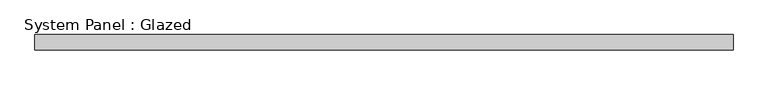
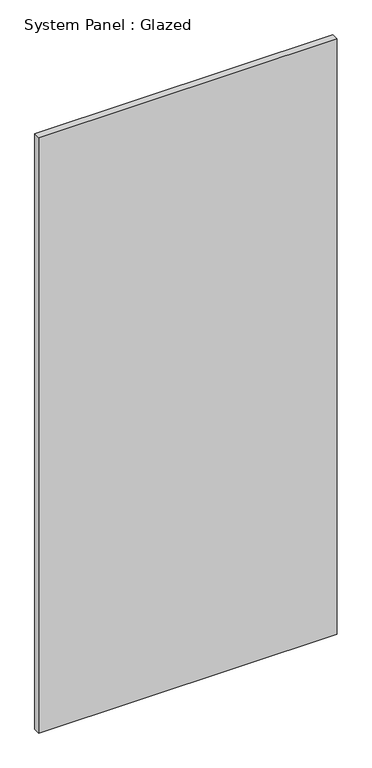
"""IFC4 building model written with IfcOpenShell, lengths in millimetres: plate geometry, System Panel : Glazed."""

from ifc_helpers import new_model, si_unit, origin, origin_with_axes, place, context, project, spatial, polyline, outline, extrude, source, transform, mapped, element, save


def system_panel_glazed_cac99656(model_context):
    return source(origin(), model_context, "Body", "SweptSolid", [
        extrude(outline(polyline([(568.8031523, 24.5), (-568.8031523, 24.5), (-568.8031523, 49.5), (568.8031523, 49.5), (568.8031523, 24.5)])), origin_with_axes(), (0.0, 0.0, 1.0), 2400.0),
    ])


if __name__ == "__main__":
    model = new_model("IFC4")
    model_context = context("Model", 3, world=origin())
    ifc_project = project(units=[si_unit("LENGTHUNIT", "METRE", prefix="MILLI")], contexts=[model_context])
    site = spatial("IfcSite", under=ifc_project)
    building = spatial("IfcBuilding", under=site)
    placement = place(None, origin())
    system_panel_glazed_shape = system_panel_glazed_cac99656(model_context)
    element("IfcPlate", 1, ObjectType="System Panel : Glazed", at=placement, inside=building, context=model_context, shape_type="MappedRepresentation", body=[
        mapped(system_panel_glazed_shape, transform((0.0, 0.0, 0.0), x_axis=(1.0, 0.0, 0.0), y_axis=(0.0, 1.0, 0.0), z_axis=(0.0, 0.0, 1.0))),
    ])
    save(model, "model.ifc")

# Revit data of these elements
# Type "System Panel : Glazed"
#   Keynote = "H11"
#   Construction Type Id = "GSP4R"
#   Analytic Construction = "1/8 in Pilkington single glazing"
#   Visual Light Transmittance = 0.9
#   Solar Heat Gain Coefficient = 0.86
#   Heat Transfer Coefficient (U) = 6.7069 W/(m²·K)
#   Define Thermal Properties by = 1
# Element 1 (IfcPlate, "System Panel : Glazed")
#   Materials on its faces: "Glass"
# Materials
#   "Glass": class "Glass", colour RGB 0 128 192, transparency 0.9, Description = "Soda Lime Glass", Cost = 0
